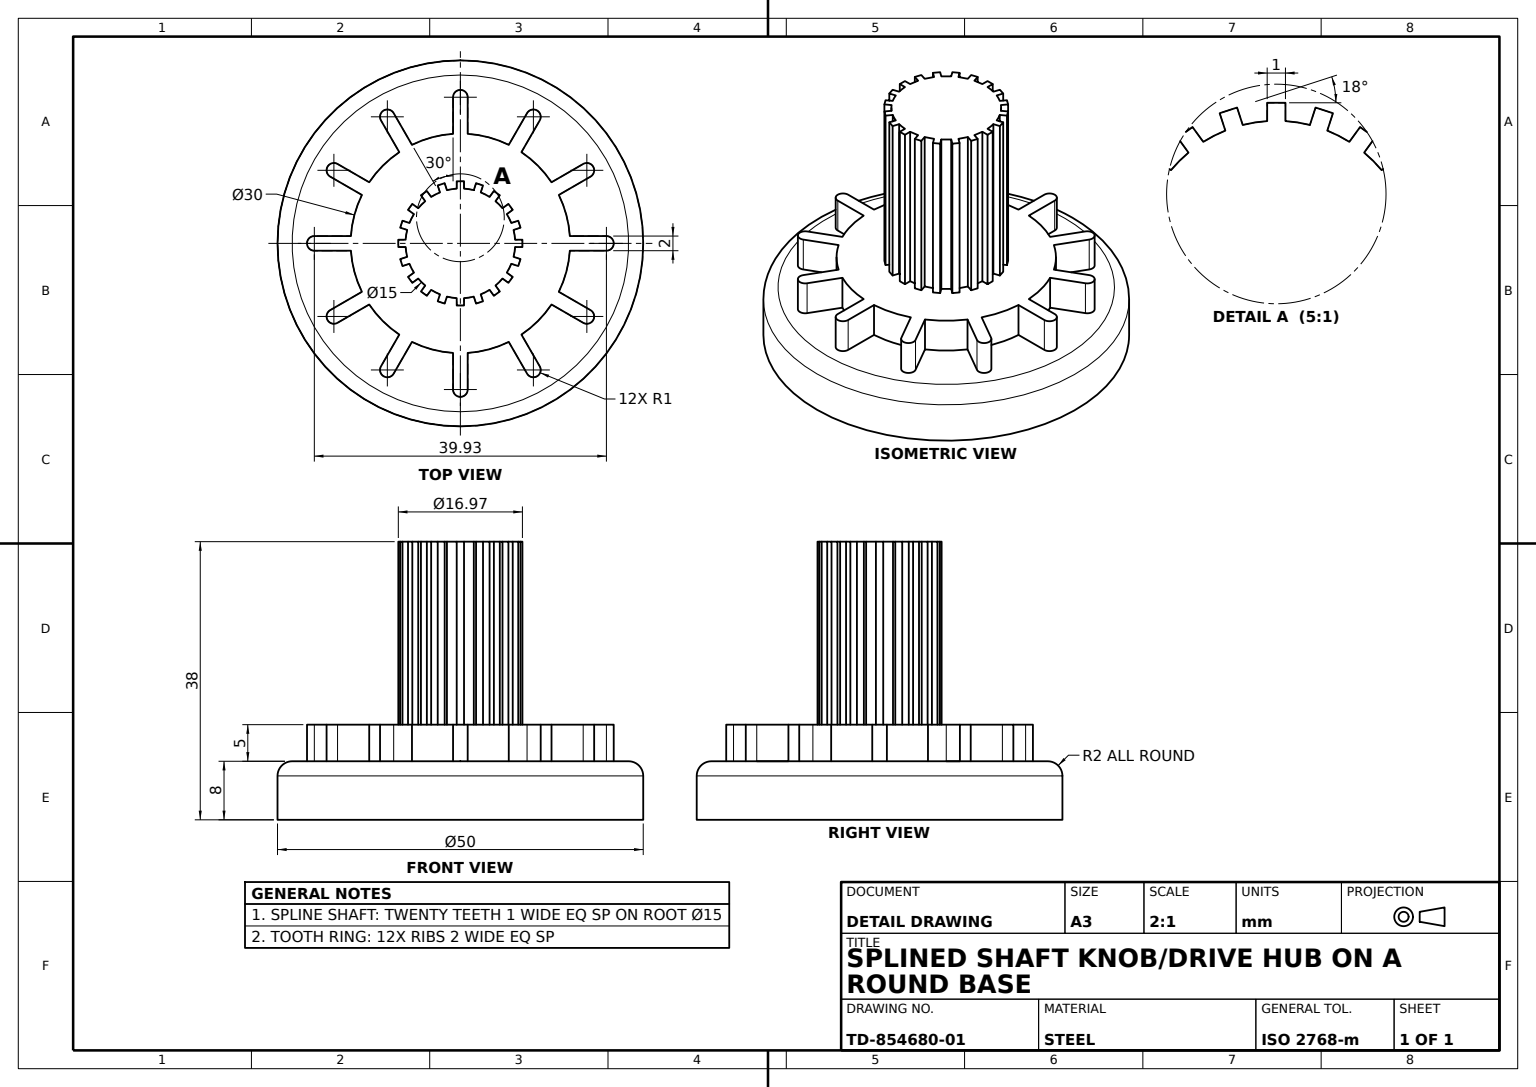
from build123d import *

# Parameters (mm, degrees)
BASE_DISC_SKETCH_R        = 25
BASE_DISC_50_DEPTH        = 8
TOOTH_RING_12T_30_DEPTH   = 5
SPLINE_SHAFT_20T_15_DEPTH = 25
BASE_EDGE_FILLET_R2_R     = 2


with BuildPart() as part:
    # Base Disc Sketch → Base Disc Ø50 (new body)
    with BuildSketch(Plane(origin=(0, 0, 0), x_dir=(1, 0, 0), z_dir=(0, 1, 0))):
        with Locations(Location((0, 0, 0), (0, 0, 270))):
            Circle(BASE_DISC_SKETCH_R)
    extrude(amount=BASE_DISC_50_DEPTH)

    # Tooth Ring Sketch → Tooth Ring 12T Ø30 (add)
    with BuildSketch(Plane(origin=(0, 8, 0), x_dir=(1, 0, 0), z_dir=(0, 1, 0))):
        with BuildLine():
            Line((8.349340177, 12.461481397), (10.849340177, 16.791608416))
            ThreePointArc((10.849340177, 16.791608416), (10.483314774, 18.15763382), (9.11728937, 17.791608416))
            Line((9.11728937, 17.791608416), (6.61728937, 13.461481397))
            ThreePointArc((6.61728937, 13.461481397), (3.882285677, 14.488887394), (1, 14.966629547))
            Line((1, 14.966629547), (1, 19.966629547))
            ThreePointArc((1, 19.966629547), (0, 20.966629547), (-1, 19.966629547))
            Line((-1, 19.966629547), (-1, 14.966629547))
            ThreePointArc((-1, 14.966629547), (-3.882285677, 14.488887394), (-6.61728937, 13.461481397))
            Line((-6.61728937, 13.461481397), (-9.11728937, 17.791608416))
            ThreePointArc((-9.11728937, 17.791608416), (-10.483314774, 18.15763382), (-10.849340177, 16.791608416))
            Line((-10.849340177, 16.791608416), (-8.349340177, 12.461481397))
            ThreePointArc((-8.349340177, 12.461481397), (-10.606601718, 10.606601718), (-12.461481397, 8.349340177))
            Line((-12.461481397, 8.349340177), (-16.791608416, 10.849340177))
            ThreePointArc((-16.791608416, 10.849340177), (-18.15763382, 10.483314774), (-17.791608416, 9.11728937))
            Line((-17.791608416, 9.11728937), (-13.461481397, 6.61728937))
            ThreePointArc((-13.461481397, 6.61728937), (-14.488887394, 3.882285677), (-14.966629547, 1))
            Line((-14.966629547, 1), (-19.966629547, 1))
            ThreePointArc((-19.966629547, 1), (-20.966629547, 0), (-19.966629547, -1))
            Line((-19.966629547, -1), (-14.966629547, -1))
            ThreePointArc((-14.966629547, -1), (-14.488887394, -3.882285677), (-13.461481397, -6.61728937))
            Line((-13.461481397, -6.61728937), (-17.791608416, -9.11728937))
            ThreePointArc((-17.791608416, -9.11728937), (-18.15763382, -10.483314774), (-16.791608416, -10.849340177))
            Line((-16.791608416, -10.849340177), (-12.461481397, -8.349340177))
            ThreePointArc((-12.461481397, -8.349340177), (-10.606601718, -10.606601718), (-8.349340177, -12.461481397))
            Line((-8.349340177, -12.461481397), (-10.849340177, -16.791608416))
            ThreePointArc((-10.849340177, -16.791608416), (-10.483314774, -18.15763382), (-9.11728937, -17.791608416))
            Line((-9.11728937, -17.791608416), (-6.61728937, -13.461481397))
            ThreePointArc((-6.61728937, -13.461481397), (-3.882285677, -14.488887394), (-1, -14.966629547))
            Line((-1, -14.966629547), (-1, -19.966629547))
            ThreePointArc((-1, -19.966629547), (0, -20.966629547), (1, -19.966629547))
            Line((1, -19.966629547), (1, -14.966629547))
            ThreePointArc((1, -14.966629547), (3.882285677, -14.488887394), (6.61728937, -13.461481397))
            Line((6.61728937, -13.461481397), (9.11728937, -17.791608416))
            ThreePointArc((9.11728937, -17.791608416), (10.483314774, -18.15763382), (10.849340177, -16.791608416))
            Line((10.849340177, -16.791608416), (8.349340177, -12.461481397))
            ThreePointArc((8.349340177, -12.461481397), (10.606601718, -10.606601718), (12.461481397, -8.349340177))
            Line((12.461481397, -8.349340177), (16.791608416, -10.849340177))
            ThreePointArc((16.791608416, -10.849340177), (18.15763382, -10.483314774), (17.791608416, -9.11728937))
            Line((17.791608416, -9.11728937), (13.461481397, -6.61728937))
            ThreePointArc((13.461481397, -6.61728937), (14.488887394, -3.882285677), (14.966629547, -1))
            Line((14.966629547, -1), (19.966629547, -1))
            ThreePointArc((19.966629547, -1), (20.966629547, 0), (19.966629547, 1))
            Line((19.966629547, 1), (14.966629547, 1))
            ThreePointArc((14.966629547, 1), (14.488887394, 3.882285677), (13.461481397, 6.61728937))
            Line((13.461481397, 6.61728937), (17.791608416, 9.11728937))
            ThreePointArc((17.791608416, 9.11728937), (18.15763382, 10.483314774), (16.791608416, 10.849340177))
            Line((16.791608416, 10.849340177), (12.461481397, 8.349340177))
            ThreePointArc((12.461481397, 8.349340177), (10.606601718, 10.606601718), (8.349340177, 12.461481397))
        make_face()
    extrude(amount=TOOTH_RING_12T_30_DEPTH)

    # Spline Shaft Sketch → Spline Shaft 20T Ø15 (add)
    with BuildSketch(Plane(origin=(0, 13, 0), x_dir=(1, 0, 0), z_dir=(0, 1, 0))):
        with BuildLine():
            Line((1.836943181, 7.271563776), (2.145960176, 8.222620292))
            Line((2.145960176, 8.222620292), (3.097016692, 7.913603298))
            Line((3.097016692, 7.913603298), (2.787999697, 6.962546782))
            ThreePointArc((2.787999697, 6.962546782), (3.404928748, 6.682548931), (3.994073565, 6.348021452))
            Line((3.994073565, 6.348021452), (4.581858817, 7.157038447))
            Line((4.581858817, 7.157038447), (5.390875812, 6.569253194))
            Line((5.390875812, 6.569253194), (4.803090559, 5.7602362))
            ThreePointArc((4.803090559, 5.7602362), (5.303300859, 5.303300859), (5.7602362, 4.803090559))
            Line((5.7602362, 4.803090559), (6.569253194, 5.390875812))
            Line((6.569253194, 5.390875812), (7.157038447, 4.581858817))
            Line((7.157038447, 4.581858817), (6.348021452, 3.994073565))
            ThreePointArc((6.348021452, 3.994073565), (6.682548931, 3.404928748), (6.962546782, 2.787999697))
            Line((6.962546782, 2.787999697), (7.913603298, 3.097016692))
            Line((7.913603298, 3.097016692), (8.222620292, 2.145960176))
            Line((8.222620292, 2.145960176), (7.271563776, 1.836943181))
            ThreePointArc((7.271563776, 1.836943181), (7.407662554, 1.173258488), (7.483314774, 0.5))
            Line((7.483314774, 0.5), (8.483314774, 0.5))
            Line((8.483314774, 0.5), (8.483314774, -0.5))
            Line((8.483314774, -0.5), (7.483314774, -0.5))
            ThreePointArc((7.483314774, -0.5), (7.407662554, -1.173258488), (7.271563776, -1.836943181))
            Line((7.271563776, -1.836943181), (8.222620292, -2.145960176))
            Line((8.222620292, -2.145960176), (7.913603298, -3.097016692))
            Line((7.913603298, -3.097016692), (6.962546782, -2.787999697))
            ThreePointArc((6.962546782, -2.787999697), (6.682548931, -3.404928748), (6.348021452, -3.994073565))
            Line((6.348021452, -3.994073565), (7.157038447, -4.581858817))
            Line((7.157038447, -4.581858817), (6.569253194, -5.390875812))
            Line((6.569253194, -5.390875812), (5.7602362, -4.803090559))
            ThreePointArc((5.7602362, -4.803090559), (5.303300859, -5.303300859), (4.803090559, -5.7602362))
            Line((4.803090559, -5.7602362), (5.390875812, -6.569253194))
            Line((5.390875812, -6.569253194), (4.581858817, -7.157038447))
            Line((4.581858817, -7.157038447), (3.994073565, -6.348021452))
            ThreePointArc((3.994073565, -6.348021452), (3.404928748, -6.682548931), (2.787999697, -6.962546782))
            Line((2.787999697, -6.962546782), (3.097016692, -7.913603298))
            Line((3.097016692, -7.913603298), (2.145960176, -8.222620292))
            Line((2.145960176, -8.222620292), (1.836943181, -7.271563776))
            ThreePointArc((1.836943181, -7.271563776), (1.173258488, -7.407662554), (0.5, -7.483314774))
            Line((0.5, -7.483314774), (0.5, -8.483314774))
            Line((0.5, -8.483314774), (-0.5, -8.483314774))
            Line((-0.5, -8.483314774), (-0.5, -7.483314774))
            ThreePointArc((-0.5, -7.483314774), (-1.173258488, -7.407662554), (-1.836943181, -7.271563776))
            Line((-1.836943181, -7.271563776), (-2.145960176, -8.222620292))
            Line((-2.145960176, -8.222620292), (-3.097016692, -7.913603298))
            Line((-3.097016692, -7.913603298), (-2.787999697, -6.962546782))
            ThreePointArc((-2.787999697, -6.962546782), (-3.404928748, -6.682548931), (-3.994073565, -6.348021452))
            Line((-3.994073565, -6.348021452), (-4.581858817, -7.157038447))
            Line((-4.581858817, -7.157038447), (-5.390875812, -6.569253194))
            Line((-5.390875812, -6.569253194), (-4.803090559, -5.7602362))
            ThreePointArc((-4.803090559, -5.7602362), (-5.303300859, -5.303300859), (-5.7602362, -4.803090559))
            Line((-5.7602362, -4.803090559), (-6.569253194, -5.390875812))
            Line((-6.569253194, -5.390875812), (-7.157038447, -4.581858817))
            Line((-7.157038447, -4.581858817), (-6.348021452, -3.994073565))
            ThreePointArc((-6.348021452, -3.994073565), (-6.682548931, -3.404928748), (-6.962546782, -2.787999697))
            Line((-6.962546782, -2.787999697), (-7.913603298, -3.097016692))
            Line((-7.913603298, -3.097016692), (-8.222620292, -2.145960176))
            Line((-8.222620292, -2.145960176), (-7.271563776, -1.836943181))
            ThreePointArc((-7.271563776, -1.836943181), (-7.407662554, -1.173258488), (-7.483314774, -0.5))
            Line((-7.483314774, -0.5), (-8.483314774, -0.5))
            Line((-8.483314774, -0.5), (-8.483314774, 0.5))
            Line((-8.483314774, 0.5), (-7.483314774, 0.5))
            ThreePointArc((-7.483314774, 0.5), (-7.407662554, 1.173258488), (-7.271563776, 1.836943181))
            Line((-7.271563776, 1.836943181), (-8.222620292, 2.145960176))
            Line((-8.222620292, 2.145960176), (-7.913603298, 3.097016692))
            Line((-7.913603298, 3.097016692), (-6.962546782, 2.787999697))
            ThreePointArc((-6.962546782, 2.787999697), (-6.682548931, 3.404928748), (-6.348021452, 3.994073565))
            Line((-6.348021452, 3.994073565), (-7.157038447, 4.581858817))
            Line((-7.157038447, 4.581858817), (-6.569253194, 5.390875812))
            Line((-6.569253194, 5.390875812), (-5.7602362, 4.803090559))
            ThreePointArc((-5.7602362, 4.803090559), (-5.303300859, 5.303300859), (-4.803090559, 5.7602362))
            Line((-4.803090559, 5.7602362), (-5.390875812, 6.569253194))
            Line((-5.390875812, 6.569253194), (-4.581858817, 7.157038447))
            Line((-4.581858817, 7.157038447), (-3.994073565, 6.348021452))
            ThreePointArc((-3.994073565, 6.348021452), (-3.404928748, 6.682548931), (-2.787999697, 6.962546782))
            Line((-2.787999697, 6.962546782), (-3.097016692, 7.913603298))
            Line((-3.097016692, 7.913603298), (-2.145960176, 8.222620292))
            Line((-2.145960176, 8.222620292), (-1.836943181, 7.271563776))
            ThreePointArc((-1.836943181, 7.271563776), (-1.173258488, 7.407662554), (-0.5, 7.483314774))
            Line((-0.5, 7.483314774), (-0.5, 8.483314774))
            Line((-0.5, 8.483314774), (0.5, 8.483314774))
            Line((0.5, 8.483314774), (0.5, 7.483314774))
            ThreePointArc((0.5, 7.483314774), (1.173258488, 7.407662554), (1.836943181, 7.271563776))
        make_face()
    extrude(amount=SPLINE_SHAFT_20T_15_DEPTH)

    # Base Edge Fillet R2
    base_edge_fillet_r2_edges = [part.edges().sort_by_distance(p)[0] for p in [
        (0, 8, -25),
    ]]
    fillet(base_edge_fillet_r2_edges, radius=BASE_EDGE_FILLET_R2_R)


solid = part.part
